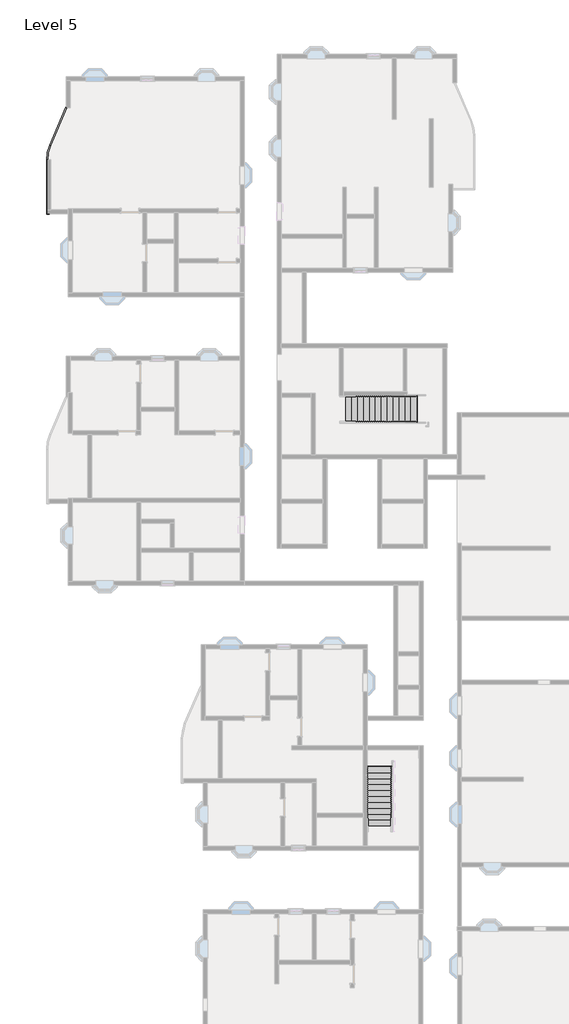
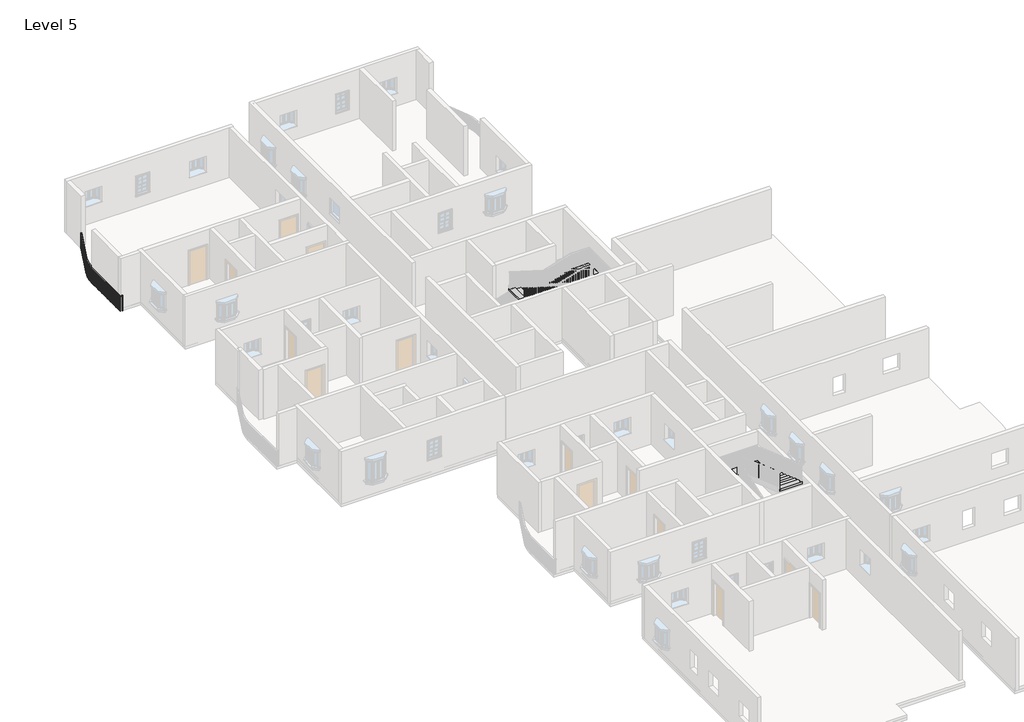
# One storey, part 12 of 14: 2 stair flights, 1 railing.
"""IFC4 building model written with IfcOpenShell, lengths in millimetres."""

from ifc_helpers import new_model, si_unit, frame, origin, place, context, project, spatial, polyline, circle_curve, outline, extrude, transform, mapped, element, save
from ifc_brep_helpers import plane_surface, cylinder_surface, revolved_surface, advanced_brep
from components import stair_flight_04159850, stair_flight_0dc38caa

model = new_model("IFC4")

# Units and contexts
model_context = context("Model", 3, world=origin())
ifc_project = project(units=[si_unit("LENGTHUNIT", "METRE", prefix="MILLI")], contexts=[model_context])

# Site, building, storey
site = spatial("IfcSite", under=ifc_project)
building = spatial("IfcBuilding", under=site)
storey = spatial("IfcBuildingStorey", under=building, Name="Level 5", Elevation=12192.0)

# Railing
placement = place(None, origin())
element("IfcRailing", 1, ObjectType="Handrail - Rectangular", at=placement, inside=storey, context=model_context, shape_type="SolidModel", body=[
    advanced_brep(
    [(-19327.739878, 27355.8257339, 13106.4), (-19327.739878, 27355.8257339, 13055.6), (-19374.4383922, 27375.822953, 13055.6), (-19374.4383922, 27375.822953, 13106.4), (-20162.483418, 25406.4905323, 13106.4), (-20162.483418, 25406.4905323, 13055.6), (-20209.1819322, 25426.4877514, 13055.6), (-20209.1819322, 25426.4877514, 13106.4), (-20316.2891351, 24656.5948172, 13055.6), (-20316.2891351, 24656.5948172, 13106.4), (-20367.0891351, 24656.5948172, 13055.6), (-20367.0891351, 24656.5948172, 13106.4), (-20316.2891351, 21915.0583494, 13106.4), (-20316.2891351, 21915.0583494, 13055.6), (-20367.0891351, 21864.2583494, 13055.6), (-20367.0891351, 21864.2583494, 13106.4), (-20240.0891351, 21915.0583494, 13106.4), (-20240.0891351, 21864.2583494, 13106.4), (-20240.0891351, 21864.2583494, 13055.6), (-20240.0891351, 21915.0583494, 13055.6)],
    [
        (0, 1),
        (1, 2),
        (2, 3),
        (3, 0),
        (0, 4),
        (4, 5),
        (5, 1),
        (5, 6),
        (6, 2),
        (6, 7),
        (7, 3),
        (7, 4),
        (8, 5, circle_curve(frame((-18411.2891351, 24656.5948172, 13055.6), z_axis=(0.0, 0.0, -1.0), x_axis=(-0.9192620907623792, 0.3936460446736121, 0.0)), 1905.0)),
        (4, 9, circle_curve(frame((-18411.2891351, 24656.5948172, 13106.4), z_axis=(0.0, 0.0, 1.0), x_axis=(-0.9192620907623792, 0.3936460446736121, 0.0)), 1905.0)),
        (9, 8),
        (10, 6, circle_curve(frame((-18411.2891351, 24656.5948172, 13055.6), z_axis=(0.0, 0.0, -1.0), x_axis=(-0.9192620907623792, 0.3936460446736121, 0.0)), 1955.8)),
        (8, 10),
        (11, 7, circle_curve(frame((-18411.2891351, 24656.5948172, 13106.4), z_axis=(0.0, 0.0, -1.0), x_axis=(-0.9192620907623792, 0.3936460446736121, 0.0)), 1955.8)),
        (10, 11),
        (11, 9),
        (9, 12),
        (12, 13),
        (13, 8),
        (13, 14),
        (14, 10),
        (14, 15),
        (15, 11),
        (15, 12),
        (16, 17),
        (17, 18),
        (18, 19),
        (19, 16),
        (12, 16),
        (19, 13),
        (18, 14),
        (17, 15),
    ],
    [
        plane_surface(frame((-19351.0891351, 27365.8243434, 13106.4), z_axis=(0.3936460446736102, 0.91926209076238, 0.0), x_axis=(0.91926209076238, -0.3936460446736102, 0.0))),
        plane_surface(frame((-19327.739878, 27355.8257339, 13106.4), z_axis=(0.91926209076238, -0.3936460446736102, 0.0), x_axis=(-0.3936460446736102, -0.91926209076238, 0.0))),
        plane_surface(frame((-19327.739878, 27355.8257339, 13055.6), z_axis=(0.0, 0.0, -1.0), x_axis=(-0.3936460446736102, -0.91926209076238, 0.0))),
        plane_surface(frame((-19374.4383922, 27375.822953, 13055.6), z_axis=(-0.91926209076238, 0.3936460446736102, 0.0), x_axis=(-0.3936460446736102, -0.91926209076238, 0.0))),
        plane_surface(frame((-19374.4383922, 27375.822953, 13106.4), z_axis=(0.0, 0.0, 1.0), x_axis=(-0.3936460446736102, -0.91926209076238, 0.0))),
        revolved_surface(polyline([(-20162.48341800233, 25406.49053230323, 13106.4), (-20162.48341800233, 25406.49053230323, 13055.6)]), (-18411.2891351, 24656.5948172, 13106.4), (0.0, 0.0, 1.0)),
        plane_surface(frame((-18411.2891351, 24656.5948172, 13055.6), z_axis=(0.0, 0.0, -1.0), x_axis=(-0.9192620907623792, 0.3936460446736121, 0.0))),
        cylinder_surface(frame((-18411.2891351, 24656.5948172, 13106.4), z_axis=(0.0, 0.0, 1.0), x_axis=(-0.9192620907623792, 0.3936460446736121, 0.0)), 1955.8),
        plane_surface(frame((-18411.2891351, 24656.5948172, 13106.4), z_axis=(0.0, 0.0, 1.0), x_axis=(-0.9192620907623792, 0.3936460446736121, 0.0))),
        plane_surface(frame((-20316.2891351, 24656.5948172, 13106.4), z_axis=(1.0, 0.0, 0.0), x_axis=(0.0, -1.0, 0.0))),
        plane_surface(frame((-20316.2891351, 24656.5948172, 13055.6), z_axis=(0.0, 0.0, -1.0), x_axis=(0.0, -1.0, 0.0))),
        plane_surface(frame((-20367.0891351, 24656.5948172, 13055.6), z_axis=(-1.0, 0.0, 0.0), x_axis=(0.0, -1.0, 0.0))),
        plane_surface(frame((-20367.0891351, 24656.5948172, 13106.4), z_axis=(0.0, 0.0, 1.0), x_axis=(0.0, -1.0, 0.0))),
        plane_surface(frame((-20240.0891351, 21889.6583494, 13106.4), z_axis=(1.0, 0.0, 0.0), x_axis=(0.0, 1.0, 0.0))),
        plane_surface(frame((-20316.2891351, 21915.0583494, 13106.4), z_axis=(0.0, 1.0, 0.0), x_axis=(1.0, 0.0, 0.0))),
        plane_surface(frame((-20316.2891351, 21915.0583494, 13055.6), z_axis=(0.0, 0.0, -1.0), x_axis=(1.0, 0.0, 0.0))),
        plane_surface(frame((-20367.0891351, 21864.2583494, 13055.6), z_axis=(0.0, -1.0, 0.0), x_axis=(1.0, 0.0, 0.0))),
        plane_surface(frame((-20367.0891351, 21864.2583494, 13106.4), z_axis=(0.0, 0.0, 1.0), x_axis=(1.0, 0.0, 0.0))),
    ],
    [
        (0, [[1, 2, 3, 4]]),
        (1, [[-1, 5, 6, 7]]),
        (2, [[-2, -7, 8, 9]]),
        (3, [[-3, -9, 10, 11]]),
        (4, [[-4, -11, 12, -5]]),
        (5, [[13, -6, 14, 15]]),
        (6, [[16, -8, -13, 17]]),
        (7, [[18, -10, -16, 19]]),
        (8, [[-14, -12, -18, 20]]),
        (9, [[-15, 21, 22, 23]]),
        (10, [[-17, -23, 24, 25]]),
        (11, [[-19, -25, 26, 27]]),
        (12, [[-20, -27, 28, -21]]),
        (13, [[29, 30, 31, 32]]),
        (14, [[-22, 33, -32, 34]]),
        (15, [[-24, -34, -31, 35]]),
        (16, [[-26, -35, -30, 36]]),
        (17, [[-28, -36, -29, -33]]),
    ],
),
    extrude(outline(polyline([(-20351.2141351, 21922.9198172), (-20332.1641351, 21922.9198172), (-20332.1641351, 21903.8698172), (-20351.2141351, 21903.8698172), (-20351.2141351, 21922.9198172)])), frame((0.0, 0.0, 12192.0), z_axis=(0.0, 0.0, 1.0), x_axis=(1.0, 0.0, 0.0)), (0.0, 0.0, 1.0), 863.6),
    extrude(outline(polyline([(-20351.2141351, 22024.5198172), (-20332.1641351, 22024.5198172), (-20332.1641351, 22005.4698172), (-20351.2141351, 22005.4698172), (-20351.2141351, 22024.5198172)])), frame((0.0, 0.0, 12192.0), z_axis=(0.0, 0.0, 1.0), x_axis=(1.0, 0.0, 0.0)), (0.0, 0.0, 1.0), 863.6),
    extrude(outline(polyline([(-20351.2141351, 22126.1198172), (-20332.1641351, 22126.1198172), (-20332.1641351, 22107.0698172), (-20351.2141351, 22107.0698172), (-20351.2141351, 22126.1198172)])), frame((0.0, 0.0, 12192.0), z_axis=(0.0, 0.0, 1.0), x_axis=(1.0, 0.0, 0.0)), (0.0, 0.0, 1.0), 863.6),
    extrude(outline(polyline([(-20351.2141351, 22227.7198172), (-20332.1641351, 22227.7198172), (-20332.1641351, 22208.6698172), (-20351.2141351, 22208.6698172), (-20351.2141351, 22227.7198172)])), frame((0.0, 0.0, 12192.0), z_axis=(0.0, 0.0, 1.0), x_axis=(1.0, 0.0, 0.0)), (0.0, 0.0, 1.0), 863.6),
    extrude(outline(polyline([(-20351.2141351, 22329.3198172), (-20332.1641351, 22329.3198172), (-20332.1641351, 22310.2698172), (-20351.2141351, 22310.2698172), (-20351.2141351, 22329.3198172)])), frame((0.0, 0.0, 12192.0), z_axis=(0.0, 0.0, 1.0), x_axis=(1.0, 0.0, 0.0)), (0.0, 0.0, 1.0), 863.6),
    extrude(outline(polyline([(-20351.2141351, 22430.9198172), (-20332.1641351, 22430.9198172), (-20332.1641351, 22411.8698172), (-20351.2141351, 22411.8698172), (-20351.2141351, 22430.9198172)])), frame((0.0, 0.0, 12192.0), z_axis=(0.0, 0.0, 1.0), x_axis=(1.0, 0.0, 0.0)), (0.0, 0.0, 1.0), 863.6),
    extrude(outline(polyline([(-20351.2141351, 22532.5198172), (-20332.1641351, 22532.5198172), (-20332.1641351, 22513.4698172), (-20351.2141351, 22513.4698172), (-20351.2141351, 22532.5198172)])), frame((0.0, 0.0, 12192.0), z_axis=(0.0, 0.0, 1.0), x_axis=(1.0, 0.0, 0.0)), (0.0, 0.0, 1.0), 863.6),
    extrude(outline(polyline([(-20351.2141351, 22634.1198172), (-20332.1641351, 22634.1198172), (-20332.1641351, 22615.0698172), (-20351.2141351, 22615.0698172), (-20351.2141351, 22634.1198172)])), frame((0.0, 0.0, 12192.0), z_axis=(0.0, 0.0, 1.0), x_axis=(1.0, 0.0, 0.0)), (0.0, 0.0, 1.0), 863.6),
    extrude(outline(polyline([(-20351.2141351, 22735.7198172), (-20332.1641351, 22735.7198172), (-20332.1641351, 22716.6698172), (-20351.2141351, 22716.6698172), (-20351.2141351, 22735.7198172)])), frame((0.0, 0.0, 12192.0), z_axis=(0.0, 0.0, 1.0), x_axis=(1.0, 0.0, 0.0)), (0.0, 0.0, 1.0), 863.6),
    extrude(outline(polyline([(-20351.2141351, 22837.3198172), (-20332.1641351, 22837.3198172), (-20332.1641351, 22818.2698172), (-20351.2141351, 22818.2698172), (-20351.2141351, 22837.3198172)])), frame((0.0, 0.0, 12192.0), z_axis=(0.0, 0.0, 1.0), x_axis=(1.0, 0.0, 0.0)), (0.0, 0.0, 1.0), 863.6),
    extrude(outline(polyline([(-20351.2141351, 22938.9198172), (-20332.1641351, 22938.9198172), (-20332.1641351, 22919.8698172), (-20351.2141351, 22919.8698172), (-20351.2141351, 22938.9198172)])), frame((0.0, 0.0, 12192.0), z_axis=(0.0, 0.0, 1.0), x_axis=(1.0, 0.0, 0.0)), (0.0, 0.0, 1.0), 863.6),
    extrude(outline(polyline([(-20351.2141351, 23040.5198172), (-20332.1641351, 23040.5198172), (-20332.1641351, 23021.4698172), (-20351.2141351, 23021.4698172), (-20351.2141351, 23040.5198172)])), frame((0.0, 0.0, 12192.0), z_axis=(0.0, 0.0, 1.0), x_axis=(1.0, 0.0, 0.0)), (0.0, 0.0, 1.0), 863.6),
    extrude(outline(polyline([(-20351.2141351, 23142.1198172), (-20332.1641351, 23142.1198172), (-20332.1641351, 23123.0698172), (-20351.2141351, 23123.0698172), (-20351.2141351, 23142.1198172)])), frame((0.0, 0.0, 12192.0), z_axis=(0.0, 0.0, 1.0), x_axis=(1.0, 0.0, 0.0)), (0.0, 0.0, 1.0), 863.6),
    extrude(outline(polyline([(-20351.2141351, 23243.7198172), (-20332.1641351, 23243.7198172), (-20332.1641351, 23224.6698172), (-20351.2141351, 23224.6698172), (-20351.2141351, 23243.7198172)])), frame((0.0, 0.0, 12192.0), z_axis=(0.0, 0.0, 1.0), x_axis=(1.0, 0.0, 0.0)), (0.0, 0.0, 1.0), 863.6),
    extrude(outline(polyline([(-20351.2141351, 23345.3198172), (-20332.1641351, 23345.3198172), (-20332.1641351, 23326.2698172), (-20351.2141351, 23326.2698172), (-20351.2141351, 23345.3198172)])), frame((0.0, 0.0, 12192.0), z_axis=(0.0, 0.0, 1.0), x_axis=(1.0, 0.0, 0.0)), (0.0, 0.0, 1.0), 863.6),
    extrude(outline(polyline([(-20351.2141351, 23446.9198172), (-20332.1641351, 23446.9198172), (-20332.1641351, 23427.8698172), (-20351.2141351, 23427.8698172), (-20351.2141351, 23446.9198172)])), frame((0.0, 0.0, 12192.0), z_axis=(0.0, 0.0, 1.0), x_axis=(1.0, 0.0, 0.0)), (0.0, 0.0, 1.0), 863.6),
    extrude(outline(polyline([(-20351.2141351, 23548.5198172), (-20332.1641351, 23548.5198172), (-20332.1641351, 23529.4698172), (-20351.2141351, 23529.4698172), (-20351.2141351, 23548.5198172)])), frame((0.0, 0.0, 12192.0), z_axis=(0.0, 0.0, 1.0), x_axis=(1.0, 0.0, 0.0)), (0.0, 0.0, 1.0), 863.6),
    extrude(outline(polyline([(-20351.2141351, 23650.1198172), (-20332.1641351, 23650.1198172), (-20332.1641351, 23631.0698172), (-20351.2141351, 23631.0698172), (-20351.2141351, 23650.1198172)])), frame((0.0, 0.0, 12192.0), z_axis=(0.0, 0.0, 1.0), x_axis=(1.0, 0.0, 0.0)), (0.0, 0.0, 1.0), 863.6),
    extrude(outline(polyline([(-20351.2141351, 23751.7198172), (-20332.1641351, 23751.7198172), (-20332.1641351, 23732.6698172), (-20351.2141351, 23732.6698172), (-20351.2141351, 23751.7198172)])), frame((0.0, 0.0, 12192.0), z_axis=(0.0, 0.0, 1.0), x_axis=(1.0, 0.0, 0.0)), (0.0, 0.0, 1.0), 863.6),
    extrude(outline(polyline([(-20351.2141351, 23853.3198172), (-20332.1641351, 23853.3198172), (-20332.1641351, 23834.2698172), (-20351.2141351, 23834.2698172), (-20351.2141351, 23853.3198172)])), frame((0.0, 0.0, 12192.0), z_axis=(0.0, 0.0, 1.0), x_axis=(1.0, 0.0, 0.0)), (0.0, 0.0, 1.0), 863.6),
    extrude(outline(polyline([(-20351.2141351, 23954.9198172), (-20332.1641351, 23954.9198172), (-20332.1641351, 23935.8698172), (-20351.2141351, 23935.8698172), (-20351.2141351, 23954.9198172)])), frame((0.0, 0.0, 12192.0), z_axis=(0.0, 0.0, 1.0), x_axis=(1.0, 0.0, 0.0)), (0.0, 0.0, 1.0), 863.6),
    extrude(outline(polyline([(-20351.2141351, 24056.5198172), (-20332.1641351, 24056.5198172), (-20332.1641351, 24037.4698172), (-20351.2141351, 24037.4698172), (-20351.2141351, 24056.5198172)])), frame((0.0, 0.0, 12192.0), z_axis=(0.0, 0.0, 1.0), x_axis=(1.0, 0.0, 0.0)), (0.0, 0.0, 1.0), 863.6),
    extrude(outline(polyline([(-20351.2141351, 24158.1198172), (-20332.1641351, 24158.1198172), (-20332.1641351, 24139.0698172), (-20351.2141351, 24139.0698172), (-20351.2141351, 24158.1198172)])), frame((0.0, 0.0, 12192.0), z_axis=(0.0, 0.0, 1.0), x_axis=(1.0, 0.0, 0.0)), (0.0, 0.0, 1.0), 863.6),
    extrude(outline(polyline([(-20351.2141351, 24259.7198172), (-20332.1641351, 24259.7198172), (-20332.1641351, 24240.6698172), (-20351.2141351, 24240.6698172), (-20351.2141351, 24259.7198172)])), frame((0.0, 0.0, 12192.0), z_axis=(0.0, 0.0, 1.0), x_axis=(1.0, 0.0, 0.0)), (0.0, 0.0, 1.0), 863.6),
    extrude(outline(polyline([(-20351.2141351, 24361.3198172), (-20332.1641351, 24361.3198172), (-20332.1641351, 24342.2698172), (-20351.2141351, 24342.2698172), (-20351.2141351, 24361.3198172)])), frame((0.0, 0.0, 12192.0), z_axis=(0.0, 0.0, 1.0), x_axis=(1.0, 0.0, 0.0)), (0.0, 0.0, 1.0), 863.6),
    extrude(outline(polyline([(-20351.2141351, 24462.9198172), (-20332.1641351, 24462.9198172), (-20332.1641351, 24443.8698172), (-20351.2141351, 24443.8698172), (-20351.2141351, 24462.9198172)])), frame((0.0, 0.0, 12192.0), z_axis=(0.0, 0.0, 1.0), x_axis=(1.0, 0.0, 0.0)), (0.0, 0.0, 1.0), 863.6),
    extrude(outline(polyline([(-20351.2141351, 24564.5198172), (-20332.1641351, 24564.5198172), (-20332.1641351, 24545.4698172), (-20351.2141351, 24545.4698172), (-20351.2141351, 24564.5198172)])), frame((0.0, 0.0, 12192.0), z_axis=(0.0, 0.0, 1.0), x_axis=(1.0, 0.0, 0.0)), (0.0, 0.0, 1.0), 863.6),
    extrude(outline(polyline([(-20349.6005818, 24736.2720848), (-20330.5630441, 24735.5831307), (-20331.2519982, 24716.545593), (-20350.289536, 24717.2345471), (-20349.6005818, 24736.2720848)])), frame((0.0, 0.0, 12192.0), z_axis=(0.0, 0.0, 1.0), x_axis=(1.0, 0.0, 0.0)), (0.0, 0.0, 1.0), 863.6),
    extrude(outline(polyline([(-20342.724955, 24838.1310534), (-20323.750023, 24836.4415402), (-20325.4395363, 24817.4666081), (-20344.4144683, 24819.1561214), (-20342.724955, 24838.1310534)])), frame((0.0, 0.0, 12192.0), z_axis=(0.0, 0.0, 1.0), x_axis=(1.0, 0.0, 0.0)), (0.0, 0.0, 1.0), 863.6),
    extrude(outline(polyline([(-20330.5003254, 24939.4872677), (-20311.6405491, 24936.8018743), (-20314.3259425, 24917.942098), (-20333.1857188, 24920.6274914), (-20330.5003254, 24939.4872677)])), frame((0.0, 0.0, 12192.0), z_axis=(0.0, 0.0, 1.0), x_axis=(1.0, 0.0, 0.0)), (0.0, 0.0, 1.0), 863.6),
    extrude(outline(polyline([(-20312.9605484, 25040.0600272), (-20294.2681589, 25036.3861907), (-20297.9419954, 25017.6938012), (-20316.6343849, 25021.3676377), (-20312.9605484, 25040.0600272)])), frame((0.0, 0.0, 12192.0), z_axis=(0.0, 0.0, 1.0), x_axis=(1.0, 0.0, 0.0)), (0.0, 0.0, 1.0), 863.6),
    extrude(outline(polyline([(-20290.1541995, 25139.5708014), (-20271.6809643, 25134.9186963), (-20276.3330693, 25116.4454611), (-20294.8063045, 25121.0975662), (-20290.1541995, 25139.5708014)])), frame((0.0, 0.0, 12192.0), z_axis=(0.0, 0.0, 1.0), x_axis=(1.0, 0.0, 0.0)), (0.0, 0.0, 1.0), 863.6),
    extrude(outline(polyline([(-20262.1444395, 25237.7440008), (-20243.9415192, 25232.1265109), (-20249.5590091, 25213.9235906), (-20267.7619294, 25219.5410805), (-20262.1444395, 25237.7440008)])), frame((0.0, 0.0, 12192.0), z_axis=(0.0, 0.0, 1.0), x_axis=(1.0, 0.0, 0.0)), (0.0, 0.0, 1.0), 863.6),
    extrude(outline(polyline([(-20229.0088399, 25334.3077402), (-20211.1266465, 25327.7404228), (-20217.693964, 25309.8582293), (-20235.5761574, 25316.4255468), (-20229.0088399, 25334.3077402)])), frame((0.0, 0.0, 12192.0), z_axis=(0.0, 0.0, 1.0), x_axis=(1.0, 0.0, 0.0)), (0.0, 0.0, 1.0), 863.6),
    extrude(outline(polyline([(-20155.9843907, 25510.389225), (-20138.4724479, 25502.8902678), (-20145.9714051, 25485.378325), (-20163.4833479, 25492.8772822), (-20155.9843907, 25510.389225)])), frame((0.0, 0.0, 12192.0), z_axis=(0.0, 0.0, 1.0), x_axis=(1.0, 0.0, 0.0)), (0.0, 0.0, 1.0), 863.6),
    extrude(outline(polyline([(-20115.9899526, 25603.7862534), (-20098.4780098, 25596.2872963), (-20105.9769669, 25578.7753534), (-20123.4889098, 25586.2743106), (-20115.9899526, 25603.7862534)])), frame((0.0, 0.0, 12192.0), z_axis=(0.0, 0.0, 1.0), x_axis=(1.0, 0.0, 0.0)), (0.0, 0.0, 1.0), 863.6),
    extrude(outline(polyline([(-20075.9955145, 25697.1832818), (-20058.4835716, 25689.6843247), (-20065.9825288, 25672.1723818), (-20083.4944716, 25679.671339), (-20075.9955145, 25697.1832818)])), frame((0.0, 0.0, 12192.0), z_axis=(0.0, 0.0, 1.0), x_axis=(1.0, 0.0, 0.0)), (0.0, 0.0, 1.0), 863.6),
    extrude(outline(polyline([(-20036.0010763, 25790.5803103), (-20018.4891335, 25783.0813531), (-20025.9880906, 25765.5694103), (-20043.5000335, 25773.0683674), (-20036.0010763, 25790.5803103)])), frame((0.0, 0.0, 12192.0), z_axis=(0.0, 0.0, 1.0), x_axis=(1.0, 0.0, 0.0)), (0.0, 0.0, 1.0), 863.6),
    extrude(outline(polyline([(-19996.0066382, 25883.9773387), (-19978.4946954, 25876.4783815), (-19985.9936525, 25858.9664387), (-20003.5055953, 25866.4653958), (-19996.0066382, 25883.9773387)])), frame((0.0, 0.0, 12192.0), z_axis=(0.0, 0.0, 1.0), x_axis=(1.0, 0.0, 0.0)), (0.0, 0.0, 1.0), 863.6),
    extrude(outline(polyline([(-19956.0122, 25977.3743671), (-19938.5002572, 25969.8754099), (-19945.9992144, 25952.3634671), (-19963.5111572, 25959.8624243), (-19956.0122, 25977.3743671)])), frame((0.0, 0.0, 12192.0), z_axis=(0.0, 0.0, 1.0), x_axis=(1.0, 0.0, 0.0)), (0.0, 0.0, 1.0), 863.6),
    extrude(outline(polyline([(-19916.0177619, 26070.7713955), (-19898.5058191, 26063.2724384), (-19906.0047762, 26045.7604955), (-19923.5167191, 26053.2594527), (-19916.0177619, 26070.7713955)])), frame((0.0, 0.0, 12192.0), z_axis=(0.0, 0.0, 1.0), x_axis=(1.0, 0.0, 0.0)), (0.0, 0.0, 1.0), 863.6),
    extrude(outline(polyline([(-19876.0233238, 26164.1684239), (-19858.5113809, 26156.6694668), (-19866.0103381, 26139.157524), (-19883.5222809, 26146.6564811), (-19876.0233238, 26164.1684239)])), frame((0.0, 0.0, 12192.0), z_axis=(0.0, 0.0, 1.0), x_axis=(1.0, 0.0, 0.0)), (0.0, 0.0, 1.0), 863.6),
    extrude(outline(polyline([(-19836.0288856, 26257.5654524), (-19818.5169428, 26250.0664952), (-19826.0159, 26232.5545524), (-19843.5278428, 26240.0535095), (-19836.0288856, 26257.5654524)])), frame((0.0, 0.0, 12192.0), z_axis=(0.0, 0.0, 1.0), x_axis=(1.0, 0.0, 0.0)), (0.0, 0.0, 1.0), 863.6),
    extrude(outline(polyline([(-19796.0344475, 26350.9624808), (-19778.5225047, 26343.4635236), (-19786.0214618, 26325.9515808), (-19803.5334046, 26333.450538), (-19796.0344475, 26350.9624808)])), frame((0.0, 0.0, 12192.0), z_axis=(0.0, 0.0, 1.0), x_axis=(1.0, 0.0, 0.0)), (0.0, 0.0, 1.0), 863.6),
    extrude(outline(polyline([(-19756.0400094, 26444.3595092), (-19738.5280665, 26436.860552), (-19746.0270237, 26419.3486092), (-19763.5389665, 26426.8475664), (-19756.0400094, 26444.3595092)])), frame((0.0, 0.0, 12192.0), z_axis=(0.0, 0.0, 1.0), x_axis=(1.0, 0.0, 0.0)), (0.0, 0.0, 1.0), 863.6),
    extrude(outline(polyline([(-19716.0455712, 26537.7565376), (-19698.5336284, 26530.2575805), (-19706.0325855, 26512.7456376), (-19723.5445284, 26520.2445948), (-19716.0455712, 26537.7565376)])), frame((0.0, 0.0, 12192.0), z_axis=(0.0, 0.0, 1.0), x_axis=(1.0, 0.0, 0.0)), (0.0, 0.0, 1.0), 863.6),
    extrude(outline(polyline([(-19676.0511331, 26631.153566), (-19658.5391902, 26623.6546089), (-19666.0381474, 26606.1426661), (-19683.5500902, 26613.6416232), (-19676.0511331, 26631.153566)])), frame((0.0, 0.0, 12192.0), z_axis=(0.0, 0.0, 1.0), x_axis=(1.0, 0.0, 0.0)), (0.0, 0.0, 1.0), 863.6),
    extrude(outline(polyline([(-19636.0566949, 26724.5505945), (-19618.5447521, 26717.0516373), (-19626.0437093, 26699.5396945), (-19643.5556521, 26707.0386516), (-19636.0566949, 26724.5505945)])), frame((0.0, 0.0, 12192.0), z_axis=(0.0, 0.0, 1.0), x_axis=(1.0, 0.0, 0.0)), (0.0, 0.0, 1.0), 863.6),
    extrude(outline(polyline([(-19596.0622568, 26817.9476229), (-19578.550314, 26810.4486657), (-19586.0492711, 26792.9367229), (-19603.561214, 26800.4356801), (-19596.0622568, 26817.9476229)])), frame((0.0, 0.0, 12192.0), z_axis=(0.0, 0.0, 1.0), x_axis=(1.0, 0.0, 0.0)), (0.0, 0.0, 1.0), 863.6),
    extrude(outline(polyline([(-19556.0678187, 26911.3446513), (-19538.5558758, 26903.8456942), (-19546.054833, 26886.3337513), (-19563.5667758, 26893.8327085), (-19556.0678187, 26911.3446513)])), frame((0.0, 0.0, 12192.0), z_axis=(0.0, 0.0, 1.0), x_axis=(1.0, 0.0, 0.0)), (0.0, 0.0, 1.0), 863.6),
    extrude(outline(polyline([(-19516.0733805, 27004.7416797), (-19498.5614377, 26997.2427226), (-19506.0603948, 26979.7307797), (-19523.5723377, 26987.2297369), (-19516.0733805, 27004.7416797)])), frame((0.0, 0.0, 12192.0), z_axis=(0.0, 0.0, 1.0), x_axis=(1.0, 0.0, 0.0)), (0.0, 0.0, 1.0), 863.6),
    extrude(outline(polyline([(-19476.0789424, 27098.1387082), (-19458.5669996, 27090.639751), (-19466.0659567, 27073.1278082), (-19483.5778995, 27080.6267653), (-19476.0789424, 27098.1387082)])), frame((0.0, 0.0, 12192.0), z_axis=(0.0, 0.0, 1.0), x_axis=(1.0, 0.0, 0.0)), (0.0, 0.0, 1.0), 863.6),
    extrude(outline(polyline([(-19436.0845042, 27191.5357366), (-19418.5725614, 27184.0367794), (-19426.0715186, 27166.5248366), (-19443.5834614, 27174.0237937), (-19436.0845042, 27191.5357366)])), frame((0.0, 0.0, 12192.0), z_axis=(0.0, 0.0, 1.0), x_axis=(1.0, 0.0, 0.0)), (0.0, 0.0, 1.0), 863.6),
    extrude(outline(polyline([(-19396.0900661, 27284.932765), (-19378.5781233, 27277.4338078), (-19386.0770804, 27259.921865), (-19403.5890233, 27267.4208222), (-19396.0900661, 27284.932765)])), frame((0.0, 0.0, 12192.0), z_axis=(0.0, 0.0, 1.0), x_axis=(1.0, 0.0, 0.0)), (0.0, 0.0, 1.0), 863.6),
    extrude(outline(polyline([(-20351.2141351, 21899.1833494), (-20332.1641351, 21899.1833494), (-20332.1641351, 21880.1333494), (-20351.2141351, 21880.1333494), (-20351.2141351, 21899.1833494)])), frame((0.0, 0.0, 12192.0), z_axis=(0.0, 0.0, 1.0), x_axis=(1.0, 0.0, 0.0)), (0.0, 0.0, 1.0), 863.6),
    extrude(outline(polyline([(-20351.2141351, 24666.1198172), (-20332.1641351, 24666.1198172), (-20332.1641351, 24647.0698172), (-20351.2141351, 24647.0698172), (-20351.2141351, 24666.1198172)])), frame((0.0, 0.0, 12192.0), z_axis=(0.0, 0.0, 1.0), x_axis=(1.0, 0.0, 0.0)), (0.0, 0.0, 1.0), 863.6),
    extrude(outline(polyline([(-20190.839168, 25428.9945919), (-20173.3272251, 25421.4956347), (-20180.8261823, 25403.9836919), (-20198.3381251, 25411.482649), (-20190.839168, 25428.9945919)])), frame((0.0, 0.0, 12192.0), z_axis=(0.0, 0.0, 1.0), x_axis=(1.0, 0.0, 0.0)), (0.0, 0.0, 1.0), 863.6),
    extrude(outline(polyline([(-20259.1391351, 21880.1333494), (-20259.1391351, 21899.1833494), (-20240.0891351, 21899.1833494), (-20240.0891351, 21880.1333494), (-20259.1391351, 21880.1333494)])), frame((0.0, 0.0, 12192.0), z_axis=(0.0, 0.0, 1.0), x_axis=(1.0, 0.0, 0.0)), (0.0, 0.0, 1.0), 863.6),
    extrude(outline(polyline([(-19359.8451065, 27369.573822), (-19342.3331637, 27362.0748648), (-19349.8321209, 27344.562922), (-19367.3440637, 27352.0618792), (-19359.8451065, 27369.573822)])), frame((0.0, 0.0, 12192.0), z_axis=(0.0, 0.0, 1.0), x_axis=(1.0, 0.0, 0.0)), (0.0, 0.0, 1.0), 863.6),
])

# Stair flights
stair_flight_shape = stair_flight_04159850(model_context)
element("IfcStairFlight", 2, ObjectType="2\" Tread 1\" Nosing 1/4\" Riser", at=placement, inside=storey, context=model_context, shape_type="MappedRepresentation", body=[
    mapped(stair_flight_shape, transform((0.0, 0.0, 0.0), x_axis=(1.0, 0.0, 0.0), y_axis=(0.0, 1.0, 0.0), z_axis=(0.0, 0.0, 1.0))),
])
stair_flight_2_shape = stair_flight_0dc38caa(model_context)
element("IfcStairFlight", 3, ObjectType="2\" Tread 1\" Nosing 1/4\" Riser", at=placement, inside=storey, context=model_context, shape_type="MappedRepresentation", body=[
    mapped(stair_flight_2_shape, transform((0.0, 0.0, 0.0), x_axis=(1.0, 0.0, 0.0), y_axis=(0.0, 1.0, 0.0), z_axis=(0.0, 0.0, 1.0))),
])

save(model, "model.ifc")

# Revit data of these elements
# Type "Handrail - Rectangular"
#   Assembly Code = "C2010400"
#   built-in parameter 1008612 = 0.0416667 (stored number, unit not read)
#   built-in parameter 1008611 = 0.0416667 (stored number, unit not read)
#   built-in parameter 1008609 = 0.333333 (stored number, unit not read)
#   built-in parameter 1008604 = 0.166667 (stored number, unit not read)
#   built-in parameter 1008603 = 0.166667 (stored number, unit not read)
#   Railing Height = 3' - 0"
#   built-in parameter 1008630 = 2
#   built-in parameter 1008610 = 2
#   built-in parameter 1008618 = Baluster - Square : 3/4"
# Element 1 (IfcRailing, "Handrail - Rectangular")
#   Phase Created = New Construction
# Elements 2, 3 (IfcStairFlight, "2\" Tread 1\" Nosing 1/4\" Riser")
#   Phase Created = New Construction
